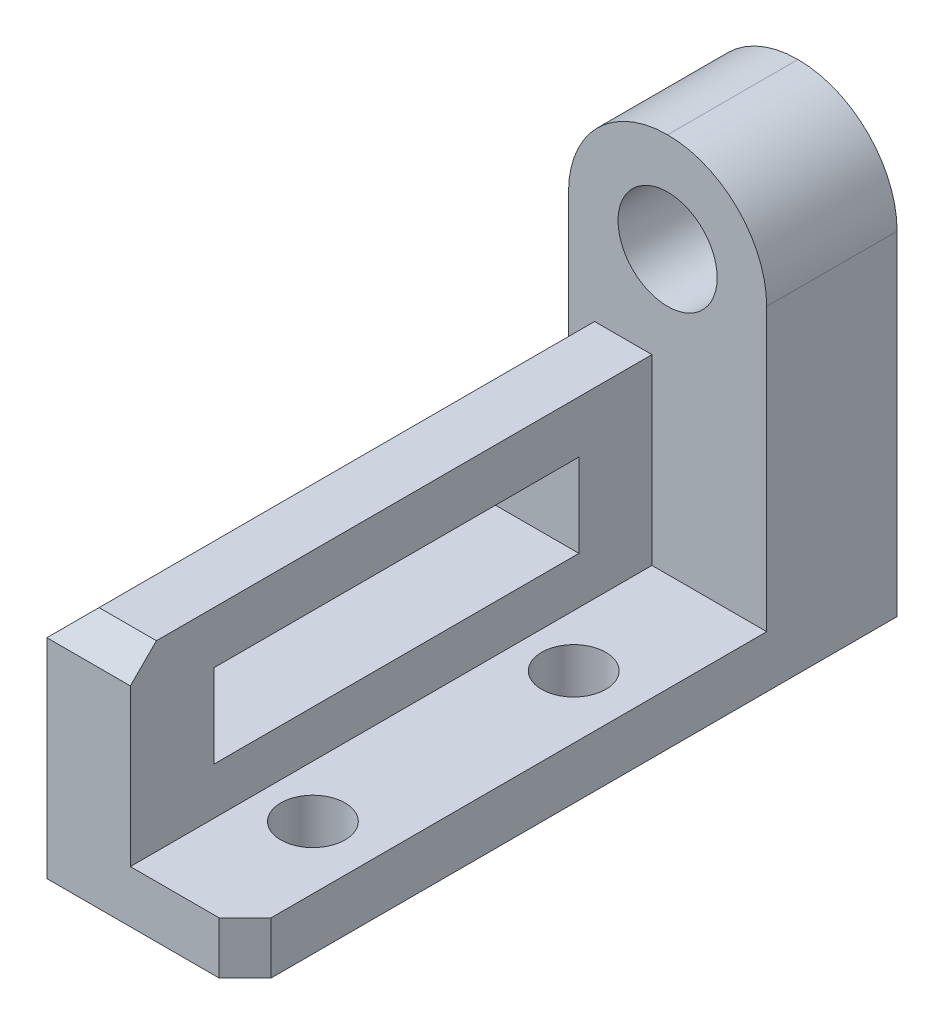
ISO-10303-21;
HEADER;
FILE_DESCRIPTION(('STEP AP214'),'2;1');
FILE_NAME('part.step','',(''),(''),'','','');
FILE_SCHEMA(('AUTOMOTIVE_DESIGN { 1 0 10303 214 1 1 1 1 }'));
ENDSEC;
DATA;
#1=APPLICATION_CONTEXT('core data for automotive mechanical design processes');
#2=APPLICATION_PROTOCOL_DEFINITION('international standard','automotive_design',2000,#1);
#3=PRODUCT_CONTEXT('',#1,'mechanical');
#4=PRODUCT('Part','Part','',(#3));
#5=PRODUCT_RELATED_PRODUCT_CATEGORY('part','',(#4));
#6=PRODUCT_DEFINITION_FORMATION('','',#4);
#7=PRODUCT_DEFINITION_CONTEXT('part definition',#1,'design');
#8=PRODUCT_DEFINITION('design','',#6,#7);
#9=PRODUCT_DEFINITION_SHAPE('','',#8);
#10=(LENGTH_UNIT() NAMED_UNIT(*) SI_UNIT(.MILLI.,.METRE.));
#11=(NAMED_UNIT(*) PLANE_ANGLE_UNIT() SI_UNIT($,.RADIAN.));
#12=(NAMED_UNIT(*) SI_UNIT($,.STERADIAN.) SOLID_ANGLE_UNIT());
#13=UNCERTAINTY_MEASURE_WITH_UNIT(LENGTH_MEASURE(1.E-05),#10,'distance_accuracy_value','');
#14=(GEOMETRIC_REPRESENTATION_CONTEXT(3) GLOBAL_UNCERTAINTY_ASSIGNED_CONTEXT((#13)) GLOBAL_UNIT_ASSIGNED_CONTEXT((#10,
#11,#12)) REPRESENTATION_CONTEXT('',''));
#15=CARTESIAN_POINT('',(0.,0.,0.));
#16=DIRECTION('',(0.,0.,1.));
#17=DIRECTION('',(1.,0.,0.));
#18=AXIS2_PLACEMENT_3D('',#15,#16,#17);
#19=CARTESIAN_POINT('',(38.,10.,-100.));
#20=DIRECTION('',(0.,0.,-1.));
#21=DIRECTION('',(-1.,0.,0.));
#22=AXIS2_PLACEMENT_3D('',#19,#20,#21);
#23=PLANE('',#22);
#24=CARTESIAN_POINT('',(19.,64.,-100.));
#25=DIRECTION('',(0.,0.,1.));
#26=DIRECTION('',(1.,0.,0.));
#27=AXIS2_PLACEMENT_3D('',#24,#25,#26);
#28=CIRCLE('',#27,9.5);
#29=CARTESIAN_POINT('',(28.5,64.,-100.));
#30=VERTEX_POINT('',#29);
#31=EDGE_CURVE('E171',#30,#30,#28,.T.);
#32=ORIENTED_EDGE('',*,*,#31,.F.);
#33=EDGE_LOOP('',(#32));
#34=FACE_BOUND('',#33,.T.);
#35=CARTESIAN_POINT('',(19.,64.,-100.));
#36=DIRECTION('',(0.,0.,-1.));
#37=DIRECTION('',(-1.,0.,0.));
#38=AXIS2_PLACEMENT_3D('',#35,#36,#37);
#39=CIRCLE('',#38,19.);
#40=CARTESIAN_POINT('',(38.,64.,-100.));
#41=VERTEX_POINT('',#40);
#42=CARTESIAN_POINT('',(19.,83.,-100.));
#43=VERTEX_POINT('',#42);
#44=EDGE_CURVE('E259',#41,#43,#39,.F.);
#45=ORIENTED_EDGE('',*,*,#44,.T.);
#46=CARTESIAN_POINT('',(19.,64.,-100.));
#47=DIRECTION('',(0.,0.,-1.));
#48=DIRECTION('',(-1.,0.,0.));
#49=AXIS2_PLACEMENT_3D('',#46,#47,#48);
#50=CIRCLE('',#49,19.);
#51=CARTESIAN_POINT('',(0.,64.,-100.));
#52=VERTEX_POINT('',#51);
#53=EDGE_CURVE('E263',#43,#52,#50,.F.);
#54=ORIENTED_EDGE('',*,*,#53,.T.);
#55=DIRECTION('',(0.,-1.,0.));
#56=VECTOR('',#55,1.);
#57=CARTESIAN_POINT('',(0.,10.,-100.));
#58=LINE('',#57,#56);
#59=CARTESIAN_POINT('',(0.,40.,-100.));
#60=VERTEX_POINT('',#59);
#61=EDGE_CURVE('E207',#52,#60,#58,.T.);
#62=ORIENTED_EDGE('',*,*,#61,.T.);
#63=DIRECTION('',(0.707106781186549,0.707106781186546,0.));
#64=VECTOR('',#63,1.);
#65=CARTESIAN_POINT('',(4.00000000000011,44.0000000000001,-100.));
#66=LINE('',#65,#64);
#67=CARTESIAN_POINT('',(5.00000000000006,45.,-100.));
#68=VERTEX_POINT('',#67);
#69=EDGE_CURVE('E260',#60,#68,#66,.T.);
#70=ORIENTED_EDGE('',*,*,#69,.T.);
#71=DIRECTION('',(-1.,0.,0.));
#72=VECTOR('',#71,1.);
#73=CARTESIAN_POINT('',(0.,45.,-100.));
#74=LINE('',#73,#72);
#75=CARTESIAN_POINT('',(16.,45.,-100.));
#76=VERTEX_POINT('',#75);
#77=EDGE_CURVE('E196',#76,#68,#74,.T.);
#78=ORIENTED_EDGE('',*,*,#77,.F.);
#79=DIRECTION('',(0.,1.,0.));
#80=VECTOR('',#79,1.);
#81=CARTESIAN_POINT('',(16.,45.,-100.));
#82=LINE('',#81,#80);
#83=CARTESIAN_POINT('',(16.,10.,-100.));
#84=VERTEX_POINT('',#83);
#85=EDGE_CURVE('E191',#84,#76,#82,.T.);
#86=ORIENTED_EDGE('',*,*,#85,.F.);
#87=DIRECTION('',(-1.,0.,0.));
#88=VECTOR('',#87,1.);
#89=CARTESIAN_POINT('',(38.,10.,-100.));
#90=LINE('',#89,#88);
#91=CARTESIAN_POINT('',(38.,10.,-100.));
#92=VERTEX_POINT('',#91);
#93=EDGE_CURVE('E230',#92,#84,#90,.T.);
#94=ORIENTED_EDGE('',*,*,#93,.F.);
#95=DIRECTION('',(0.,-1.,0.));
#96=VECTOR('',#95,1.);
#97=CARTESIAN_POINT('',(38.,10.,-100.));
#98=LINE('',#97,#96);
#99=EDGE_CURVE('E215',#41,#92,#98,.T.);
#100=ORIENTED_EDGE('',*,*,#99,.F.);
#101=EDGE_LOOP('',(#45,#54,#62,#70,#78,#86,#94,#100));
#102=FACE_BOUND('',#101,.T.);
#103=ADVANCED_FACE('F41',(#34,#102),#23,.F.);
#104=CARTESIAN_POINT('',(38.,10.,0.));
#105=DIRECTION('',(0.,-1.,0.));
#106=DIRECTION('',(0.,0.,-1.));
#107=AXIS2_PLACEMENT_3D('',#104,#105,#106);
#108=PLANE('',#107);
#109=CARTESIAN_POINT('',(26.,10.,-75.));
#110=DIRECTION('',(0.,1.,0.));
#111=DIRECTION('',(0.,0.,1.));
#112=AXIS2_PLACEMENT_3D('',#109,#110,#111);
#113=CIRCLE('',#112,6.15885509382051);
#114=CARTESIAN_POINT('',(26.,10.,-68.8411449061795));
#115=VERTEX_POINT('',#114);
#116=EDGE_CURVE('E516',#115,#115,#113,.T.);
#117=ORIENTED_EDGE('',*,*,#116,.F.);
#118=EDGE_LOOP('',(#117));
#119=FACE_BOUND('',#118,.T.);
#120=CARTESIAN_POINT('',(26.,10.,-25.));
#121=DIRECTION('',(0.,1.,0.));
#122=DIRECTION('',(0.,0.,1.));
#123=AXIS2_PLACEMENT_3D('',#120,#121,#122);
#124=CIRCLE('',#123,6.15885509382051);
#125=CARTESIAN_POINT('',(26.,10.,-18.8411449061795));
#126=VERTEX_POINT('',#125);
#127=EDGE_CURVE('E524',#126,#126,#124,.T.);
#128=ORIENTED_EDGE('',*,*,#127,.F.);
#129=EDGE_LOOP('',(#128));
#130=FACE_BOUND('',#129,.T.);
#131=DIRECTION('',(-1.,0.,0.));
#132=VECTOR('',#131,1.);
#133=CARTESIAN_POINT('',(38.,10.,0.));
#134=LINE('',#133,#132);
#135=CARTESIAN_POINT('',(33.,10.,0.));
#136=VERTEX_POINT('',#135);
#137=CARTESIAN_POINT('',(16.,10.,0.));
#138=VERTEX_POINT('',#137);
#139=EDGE_CURVE('E220',#136,#138,#134,.T.);
#140=ORIENTED_EDGE('',*,*,#139,.F.);
#141=DIRECTION('',(-0.707106781186549,0.,0.707106781186547));
#142=VECTOR('',#141,1.);
#143=CARTESIAN_POINT('',(38.,10.,-5.00000000000002));
#144=LINE('',#143,#142);
#145=CARTESIAN_POINT('',(38.,10.,-5.00000000000002));
#146=VERTEX_POINT('',#145);
#147=EDGE_CURVE('E241',#136,#146,#144,.F.);
#148=ORIENTED_EDGE('',*,*,#147,.T.);
#149=DIRECTION('',(0.,0.,1.));
#150=VECTOR('',#149,1.);
#151=CARTESIAN_POINT('',(38.,10.,0.));
#152=LINE('',#151,#150);
#153=EDGE_CURVE('E212',#92,#146,#152,.T.);
#154=ORIENTED_EDGE('',*,*,#153,.F.);
#155=ORIENTED_EDGE('',*,*,#93,.T.);
#156=DIRECTION('',(0.,0.,-1.));
#157=VECTOR('',#156,1.);
#158=CARTESIAN_POINT('',(16.,10.,38.4837628097877));
#159=LINE('',#158,#157);
#160=EDGE_CURVE('E195',#138,#84,#159,.T.);
#161=ORIENTED_EDGE('',*,*,#160,.F.);
#162=EDGE_LOOP('',(#140,#148,#154,#155,#161));
#163=FACE_BOUND('',#162,.T.);
#164=ADVANCED_FACE('F306',(#119,#130,#163),#108,.F.);
#165=CARTESIAN_POINT('',(38.,0.,0.));
#166=DIRECTION('',(0.,0.,-1.));
#167=DIRECTION('',(-1.,0.,0.));
#168=AXIS2_PLACEMENT_3D('',#165,#166,#167);
#169=PLANE('',#168);
#170=DIRECTION('',(-1.,0.,0.));
#171=VECTOR('',#170,1.);
#172=CARTESIAN_POINT('',(38.,0.,0.));
#173=LINE('',#172,#171);
#174=CARTESIAN_POINT('',(33.,0.,0.));
#175=VERTEX_POINT('',#174);
#176=CARTESIAN_POINT('',(0.,0.,0.));
#177=VERTEX_POINT('',#176);
#178=EDGE_CURVE('E232',#175,#177,#173,.T.);
#179=ORIENTED_EDGE('',*,*,#178,.F.);
#180=DIRECTION('',(0.,1.,0.));
#181=VECTOR('',#180,1.);
#182=CARTESIAN_POINT('',(33.,0.,0.));
#183=LINE('',#182,#181);
#184=EDGE_CURVE('E243',#175,#136,#183,.T.);
#185=ORIENTED_EDGE('',*,*,#184,.T.);
#186=ORIENTED_EDGE('',*,*,#139,.T.);
#187=DIRECTION('',(0.,-1.,0.));
#188=VECTOR('',#187,1.);
#189=CARTESIAN_POINT('',(16.,45.,0.));
#190=LINE('',#189,#188);
#191=CARTESIAN_POINT('',(16.,40.,0.));
#192=VERTEX_POINT('',#191);
#193=EDGE_CURVE('E193',#192,#138,#190,.T.);
#194=ORIENTED_EDGE('',*,*,#193,.F.);
#195=DIRECTION('',(-1.,0.,0.));
#196=VECTOR('',#195,1.);
#197=CARTESIAN_POINT('',(38.,40.,0.));
#198=LINE('',#197,#196);
#199=CARTESIAN_POINT('',(0.,40.,0.));
#200=VERTEX_POINT('',#199);
#201=EDGE_CURVE('E242',#192,#200,#198,.T.);
#202=ORIENTED_EDGE('',*,*,#201,.T.);
#203=DIRECTION('',(0.,-1.,0.));
#204=VECTOR('',#203,1.);
#205=CARTESIAN_POINT('',(0.,0.,0.));
#206=LINE('',#205,#204);
#207=EDGE_CURVE('E192',#200,#177,#206,.T.);
#208=ORIENTED_EDGE('',*,*,#207,.T.);
#209=EDGE_LOOP('',(#179,#185,#186,#194,#202,#208));
#210=FACE_BOUND('',#209,.T.);
#211=ADVANCED_FACE('F325',(#210),#169,.F.);
#212=CARTESIAN_POINT('',(38.,0.,0.));
#213=DIRECTION('',(0.,1.,0.));
#214=DIRECTION('',(0.,0.,1.));
#215=AXIS2_PLACEMENT_3D('',#212,#213,#214);
#216=PLANE('',#215);
#217=CARTESIAN_POINT('',(26.,0.,-75.));
#218=DIRECTION('',(0.,1.,0.));
#219=DIRECTION('',(0.,0.,1.));
#220=AXIS2_PLACEMENT_3D('',#217,#218,#219);
#221=CIRCLE('',#220,6.15885509382051);
#222=CARTESIAN_POINT('',(26.,0.,-68.8411449061795));
#223=VERTEX_POINT('',#222);
#224=EDGE_CURVE('E520',#223,#223,#221,.T.);
#225=ORIENTED_EDGE('',*,*,#224,.T.);
#226=EDGE_LOOP('',(#225));
#227=FACE_BOUND('',#226,.T.);
#228=CARTESIAN_POINT('',(26.,0.,-25.));
#229=DIRECTION('',(0.,1.,0.));
#230=DIRECTION('',(0.,0.,1.));
#231=AXIS2_PLACEMENT_3D('',#228,#229,#230);
#232=CIRCLE('',#231,6.15885509382051);
#233=CARTESIAN_POINT('',(26.,0.,-18.8411449061795));
#234=VERTEX_POINT('',#233);
#235=EDGE_CURVE('E521',#234,#234,#232,.T.);
#236=ORIENTED_EDGE('',*,*,#235,.T.);
#237=EDGE_LOOP('',(#236));
#238=FACE_BOUND('',#237,.T.);
#239=DIRECTION('',(0.,0.,-1.));
#240=VECTOR('',#239,1.);
#241=CARTESIAN_POINT('',(38.,0.,0.));
#242=LINE('',#241,#240);
#243=CARTESIAN_POINT('',(38.,0.,-5.00000000000002));
#244=VERTEX_POINT('',#243);
#245=CARTESIAN_POINT('',(38.,0.,-125.));
#246=VERTEX_POINT('',#245);
#247=EDGE_CURVE('E206',#244,#246,#242,.T.);
#248=ORIENTED_EDGE('',*,*,#247,.F.);
#249=DIRECTION('',(0.707106781186549,0.,-0.707106781186547));
#250=VECTOR('',#249,1.);
#251=CARTESIAN_POINT('',(38.,0.,-5.00000000000002));
#252=LINE('',#251,#250);
#253=EDGE_CURVE('E239',#244,#175,#252,.F.);
#254=ORIENTED_EDGE('',*,*,#253,.T.);
#255=ORIENTED_EDGE('',*,*,#178,.T.);
#256=DIRECTION('',(0.,0.,-1.));
#257=VECTOR('',#256,1.);
#258=CARTESIAN_POINT('',(0.,0.,0.));
#259=LINE('',#258,#257);
#260=CARTESIAN_POINT('',(0.,0.,-125.));
#261=VERTEX_POINT('',#260);
#262=EDGE_CURVE('E218',#177,#261,#259,.T.);
#263=ORIENTED_EDGE('',*,*,#262,.T.);
#264=DIRECTION('',(-1.,0.,0.));
#265=VECTOR('',#264,1.);
#266=CARTESIAN_POINT('',(38.,0.,-125.));
#267=LINE('',#266,#265);
#268=EDGE_CURVE('E226',#246,#261,#267,.T.);
#269=ORIENTED_EDGE('',*,*,#268,.F.);
#270=EDGE_LOOP('',(#248,#254,#255,#263,#269));
#271=FACE_BOUND('',#270,.T.);
#272=ADVANCED_FACE('F317',(#227,#238,#271),#216,.F.);
#273=CARTESIAN_POINT('',(38.,0.,-125.));
#274=DIRECTION('',(0.,0.,1.));
#275=DIRECTION('',(1.,0.,0.));
#276=AXIS2_PLACEMENT_3D('',#273,#274,#275);
#277=PLANE('',#276);
#278=CARTESIAN_POINT('',(19.,64.,-125.));
#279=DIRECTION('',(0.,0.,1.));
#280=DIRECTION('',(1.,0.,0.));
#281=AXIS2_PLACEMENT_3D('',#278,#279,#280);
#282=CIRCLE('',#281,9.5);
#283=CARTESIAN_POINT('',(28.5,64.,-125.));
#284=VERTEX_POINT('',#283);
#285=EDGE_CURVE('E185',#284,#284,#282,.T.);
#286=ORIENTED_EDGE('',*,*,#285,.T.);
#287=EDGE_LOOP('',(#286));
#288=FACE_BOUND('',#287,.T.);
#289=DIRECTION('',(0.,1.,0.));
#290=VECTOR('',#289,1.);
#291=CARTESIAN_POINT('',(0.,0.,-125.));
#292=LINE('',#291,#290);
#293=CARTESIAN_POINT('',(0.,64.,-125.));
#294=VERTEX_POINT('',#293);
#295=EDGE_CURVE('E222',#261,#294,#292,.T.);
#296=ORIENTED_EDGE('',*,*,#295,.T.);
#297=CARTESIAN_POINT('',(19.,64.,-125.));
#298=DIRECTION('',(0.,0.,1.));
#299=DIRECTION('',(1.,0.,0.));
#300=AXIS2_PLACEMENT_3D('',#297,#298,#299);
#301=CIRCLE('',#300,19.);
#302=CARTESIAN_POINT('',(19.,83.,-125.));
#303=VERTEX_POINT('',#302);
#304=EDGE_CURVE('E49',#294,#303,#301,.F.);
#305=ORIENTED_EDGE('',*,*,#304,.T.);
#306=CARTESIAN_POINT('',(19.,64.,-125.));
#307=DIRECTION('',(0.,0.,1.));
#308=DIRECTION('',(1.,0.,0.));
#309=AXIS2_PLACEMENT_3D('',#306,#307,#308);
#310=CIRCLE('',#309,19.);
#311=CARTESIAN_POINT('',(38.,64.,-125.));
#312=VERTEX_POINT('',#311);
#313=EDGE_CURVE('E268',#303,#312,#310,.F.);
#314=ORIENTED_EDGE('',*,*,#313,.T.);
#315=DIRECTION('',(0.,1.,0.));
#316=VECTOR('',#315,1.);
#317=CARTESIAN_POINT('',(38.,0.,-125.));
#318=LINE('',#317,#316);
#319=EDGE_CURVE('E208',#246,#312,#318,.T.);
#320=ORIENTED_EDGE('',*,*,#319,.F.);
#321=ORIENTED_EDGE('',*,*,#268,.T.);
#322=EDGE_LOOP('',(#296,#305,#314,#320,#321));
#323=FACE_BOUND('',#322,.T.);
#324=ADVANCED_FACE('F275',(#288,#323),#277,.F.);
#325=CARTESIAN_POINT('',(38.,0.,0.));
#326=DIRECTION('',(-1.,0.,0.));
#327=DIRECTION('',(0.,0.,1.));
#328=AXIS2_PLACEMENT_3D('',#325,#326,#327);
#329=PLANE('',#328);
#330=ORIENTED_EDGE('',*,*,#319,.T.);
#331=DIRECTION('',(0.,0.,1.));
#332=VECTOR('',#331,1.);
#333=CARTESIAN_POINT('',(38.,64.,0.));
#334=LINE('',#333,#332);
#335=EDGE_CURVE('E11',#312,#41,#334,.T.);
#336=ORIENTED_EDGE('',*,*,#335,.T.);
#337=ORIENTED_EDGE('',*,*,#99,.T.);
#338=ORIENTED_EDGE('',*,*,#153,.T.);
#339=DIRECTION('',(0.,-1.,0.));
#340=VECTOR('',#339,1.);
#341=CARTESIAN_POINT('',(38.,0.,-5.00000000000002));
#342=LINE('',#341,#340);
#343=EDGE_CURVE('E237',#146,#244,#342,.T.);
#344=ORIENTED_EDGE('',*,*,#343,.T.);
#345=ORIENTED_EDGE('',*,*,#247,.T.);
#346=EDGE_LOOP('',(#330,#336,#337,#338,#344,#345));
#347=FACE_BOUND('',#346,.T.);
#348=ADVANCED_FACE('F315',(#347),#329,.F.);
#349=CARTESIAN_POINT('',(0.,0.,0.));
#350=DIRECTION('',(-1.,0.,0.));
#351=DIRECTION('',(0.,0.,1.));
#352=AXIS2_PLACEMENT_3D('',#349,#350,#351);
#353=PLANE('',#352);
#354=DIRECTION('',(0.,-1.,0.));
#355=VECTOR('',#354,1.);
#356=CARTESIAN_POINT('',(0.,35.,-16.));
#357=LINE('',#356,#355);
#358=CARTESIAN_POINT('',(0.,35.,-16.));
#359=VERTEX_POINT('',#358);
#360=CARTESIAN_POINT('',(0.,19.,-16.));
#361=VERTEX_POINT('',#360);
#362=EDGE_CURVE('E153',#359,#361,#357,.T.);
#363=ORIENTED_EDGE('',*,*,#362,.T.);
#364=DIRECTION('',(0.,0.,-1.));
#365=VECTOR('',#364,1.);
#366=CARTESIAN_POINT('',(0.,19.,-16.));
#367=LINE('',#366,#365);
#368=CARTESIAN_POINT('',(0.,19.,-86.));
#369=VERTEX_POINT('',#368);
#370=EDGE_CURVE('E165',#361,#369,#367,.T.);
#371=ORIENTED_EDGE('',*,*,#370,.T.);
#372=DIRECTION('',(0.,1.,0.));
#373=VECTOR('',#372,1.);
#374=CARTESIAN_POINT('',(0.,35.,-86.));
#375=LINE('',#374,#373);
#376=CARTESIAN_POINT('',(0.,35.,-86.));
#377=VERTEX_POINT('',#376);
#378=EDGE_CURVE('E60',#369,#377,#375,.T.);
#379=ORIENTED_EDGE('',*,*,#378,.T.);
#380=DIRECTION('',(0.,0.,1.));
#381=VECTOR('',#380,1.);
#382=CARTESIAN_POINT('',(0.,35.,-16.));
#383=LINE('',#382,#381);
#384=EDGE_CURVE('E157',#377,#359,#383,.T.);
#385=ORIENTED_EDGE('',*,*,#384,.T.);
#386=EDGE_LOOP('',(#363,#371,#379,#385));
#387=FACE_BOUND('',#386,.T.);
#388=ORIENTED_EDGE('',*,*,#61,.F.);
#389=DIRECTION('',(0.,0.,1.));
#390=VECTOR('',#389,1.);
#391=CARTESIAN_POINT('',(0.,64.,-125.));
#392=LINE('',#391,#390);
#393=EDGE_CURVE('E264',#52,#294,#392,.F.);
#394=ORIENTED_EDGE('',*,*,#393,.T.);
#395=ORIENTED_EDGE('',*,*,#295,.F.);
#396=ORIENTED_EDGE('',*,*,#262,.F.);
#397=ORIENTED_EDGE('',*,*,#207,.F.);
#398=DIRECTION('',(0.,0.,-1.));
#399=VECTOR('',#398,1.);
#400=CARTESIAN_POINT('',(0.,40.,-100.));
#401=LINE('',#400,#399);
#402=EDGE_CURVE('E255',#200,#60,#401,.T.);
#403=ORIENTED_EDGE('',*,*,#402,.T.);
#404=EDGE_LOOP('',(#388,#394,#395,#396,#397,#403));
#405=FACE_BOUND('',#404,.T.);
#406=ADVANCED_FACE('F167',(#387,#405),#353,.T.);
#407=CARTESIAN_POINT('',(0.,45.,38.4837628097877));
#408=DIRECTION('',(0.,-1.,0.));
#409=DIRECTION('',(0.,0.,-1.));
#410=AXIS2_PLACEMENT_3D('',#407,#408,#409);
#411=PLANE('',#410);
#412=DIRECTION('',(0.,0.,1.));
#413=VECTOR('',#412,1.);
#414=CARTESIAN_POINT('',(5.00000000000006,45.,0.));
#415=LINE('',#414,#413);
#416=CARTESIAN_POINT('',(5.00000000000006,45.,-5.00000000000006));
#417=VERTEX_POINT('',#416);
#418=EDGE_CURVE('E249',#68,#417,#415,.T.);
#419=ORIENTED_EDGE('',*,*,#418,.T.);
#420=DIRECTION('',(1.,0.,0.));
#421=VECTOR('',#420,1.);
#422=CARTESIAN_POINT('',(0.,45.,-5.00000000000006));
#423=LINE('',#422,#421);
#424=CARTESIAN_POINT('',(16.,45.,-5.00000000000006));
#425=VERTEX_POINT('',#424);
#426=EDGE_CURVE('E250',#417,#425,#423,.T.);
#427=ORIENTED_EDGE('',*,*,#426,.T.);
#428=DIRECTION('',(0.,0.,-1.));
#429=VECTOR('',#428,1.);
#430=CARTESIAN_POINT('',(16.,45.,38.4837628097877));
#431=LINE('',#430,#429);
#432=EDGE_CURVE('E205',#425,#76,#431,.T.);
#433=ORIENTED_EDGE('',*,*,#432,.T.);
#434=ORIENTED_EDGE('',*,*,#77,.T.);
#435=EDGE_LOOP('',(#419,#427,#433,#434));
#436=FACE_BOUND('',#435,.T.);
#437=ADVANCED_FACE('F300',(#436),#411,.F.);
#438=CARTESIAN_POINT('',(16.,45.,38.4837628097877));
#439=DIRECTION('',(-1.,0.,0.));
#440=DIRECTION('',(0.,-1.,0.));
#441=AXIS2_PLACEMENT_3D('',#438,#439,#440);
#442=PLANE('',#441);
#443=DIRECTION('',(0.,0.,-1.));
#444=VECTOR('',#443,1.);
#445=CARTESIAN_POINT('',(16.,19.,-16.));
#446=LINE('',#445,#444);
#447=CARTESIAN_POINT('',(16.,19.,-16.));
#448=VERTEX_POINT('',#447);
#449=CARTESIAN_POINT('',(16.,19.,-86.));
#450=VERTEX_POINT('',#449);
#451=EDGE_CURVE('E182',#448,#450,#446,.T.);
#452=ORIENTED_EDGE('',*,*,#451,.F.);
#453=DIRECTION('',(0.,-1.,0.));
#454=VECTOR('',#453,1.);
#455=CARTESIAN_POINT('',(16.,35.,-16.));
#456=LINE('',#455,#454);
#457=CARTESIAN_POINT('',(16.,35.,-16.));
#458=VERTEX_POINT('',#457);
#459=EDGE_CURVE('E61',#458,#448,#456,.T.);
#460=ORIENTED_EDGE('',*,*,#459,.F.);
#461=DIRECTION('',(0.,0.,1.));
#462=VECTOR('',#461,1.);
#463=CARTESIAN_POINT('',(16.,35.,-16.));
#464=LINE('',#463,#462);
#465=CARTESIAN_POINT('',(16.,35.,-86.));
#466=VERTEX_POINT('',#465);
#467=EDGE_CURVE('E166',#466,#458,#464,.T.);
#468=ORIENTED_EDGE('',*,*,#467,.F.);
#469=DIRECTION('',(0.,1.,0.));
#470=VECTOR('',#469,1.);
#471=CARTESIAN_POINT('',(16.,35.,-86.));
#472=LINE('',#471,#470);
#473=EDGE_CURVE('E175',#450,#466,#472,.T.);
#474=ORIENTED_EDGE('',*,*,#473,.F.);
#475=EDGE_LOOP('',(#452,#460,#468,#474));
#476=FACE_BOUND('',#475,.T.);
#477=ORIENTED_EDGE('',*,*,#432,.F.);
#478=DIRECTION('',(0.,0.707106781186546,-0.707106781186549));
#479=VECTOR('',#478,1.);
#480=CARTESIAN_POINT('',(16.,45.,-5.00000000000006));
#481=LINE('',#480,#479);
#482=EDGE_CURVE('E252',#425,#192,#481,.F.);
#483=ORIENTED_EDGE('',*,*,#482,.T.);
#484=ORIENTED_EDGE('',*,*,#193,.T.);
#485=ORIENTED_EDGE('',*,*,#160,.T.);
#486=ORIENTED_EDGE('',*,*,#85,.T.);
#487=EDGE_LOOP('',(#477,#483,#484,#485,#486));
#488=FACE_BOUND('',#487,.T.);
#489=ADVANCED_FACE('F303',(#476,#488),#442,.F.);
#490=CARTESIAN_POINT('',(38.,0.,-5.00000000000002));
#491=DIRECTION('',(-0.707106781186546,0.,-0.707106781186548));
#492=DIRECTION('',(0.,-1.,0.));
#493=AXIS2_PLACEMENT_3D('',#490,#491,#492);
#494=PLANE('',#493);
#495=ORIENTED_EDGE('',*,*,#147,.F.);
#496=ORIENTED_EDGE('',*,*,#184,.F.);
#497=ORIENTED_EDGE('',*,*,#253,.F.);
#498=ORIENTED_EDGE('',*,*,#343,.F.);
#499=EDGE_LOOP('',(#495,#496,#497,#498));
#500=FACE_BOUND('',#499,.T.);
#501=ADVANCED_FACE('F312',(#500),#494,.F.);
#502=CARTESIAN_POINT('',(0.,40.,0.));
#503=DIRECTION('',(-0.707106781186546,0.707106781186549,0.));
#504=DIRECTION('',(0.,0.,1.));
#505=AXIS2_PLACEMENT_3D('',#502,#503,#504);
#506=PLANE('',#505);
#507=ORIENTED_EDGE('',*,*,#69,.F.);
#508=ORIENTED_EDGE('',*,*,#402,.F.);
#509=DIRECTION('',(-0.577350269189627,-0.577350269189624,0.577350269189627));
#510=VECTOR('',#509,1.);
#511=CARTESIAN_POINT('',(0.,40.,0.));
#512=LINE('',#511,#510);
#513=EDGE_CURVE('E200',#417,#200,#512,.T.);
#514=ORIENTED_EDGE('',*,*,#513,.F.);
#515=ORIENTED_EDGE('',*,*,#418,.F.);
#516=EDGE_LOOP('',(#507,#508,#514,#515));
#517=FACE_BOUND('',#516,.T.);
#518=ADVANCED_FACE('F294',(#517),#506,.T.);
#519=CARTESIAN_POINT('',(0.,45.,-5.00000000000006));
#520=DIRECTION('',(0.,-0.707106781186549,-0.707106781186546));
#521=DIRECTION('',(1.,0.,0.));
#522=AXIS2_PLACEMENT_3D('',#519,#520,#521);
#523=PLANE('',#522);
#524=ORIENTED_EDGE('',*,*,#513,.T.);
#525=ORIENTED_EDGE('',*,*,#201,.F.);
#526=ORIENTED_EDGE('',*,*,#482,.F.);
#527=ORIENTED_EDGE('',*,*,#426,.F.);
#528=EDGE_LOOP('',(#524,#525,#526,#527));
#529=FACE_BOUND('',#528,.T.);
#530=ADVANCED_FACE('F324',(#529),#523,.F.);
#531=CARTESIAN_POINT('',(19.,64.,0.));
#532=DIRECTION('',(0.,0.,1.));
#533=DIRECTION('',(1.,0.,0.));
#534=AXIS2_PLACEMENT_3D('',#531,#532,#533);
#535=CYLINDRICAL_SURFACE('',#534,19.);
#536=ORIENTED_EDGE('',*,*,#335,.F.);
#537=ORIENTED_EDGE('',*,*,#313,.F.);
#538=DIRECTION('',(0.,0.,1.));
#539=VECTOR('',#538,1.);
#540=CARTESIAN_POINT('',(19.,83.,-125.));
#541=LINE('',#540,#539);
#542=EDGE_CURVE('E44',#43,#303,#541,.F.);
#543=ORIENTED_EDGE('',*,*,#542,.F.);
#544=ORIENTED_EDGE('',*,*,#44,.F.);
#545=EDGE_LOOP('',(#536,#537,#543,#544));
#546=FACE_BOUND('',#545,.T.);
#547=ADVANCED_FACE('F43',(#546),#535,.T.);
#548=CARTESIAN_POINT('',(19.,64.,-125.));
#549=DIRECTION('',(0.,0.,-1.));
#550=DIRECTION('',(-1.,0.,0.));
#551=AXIS2_PLACEMENT_3D('',#548,#549,#550);
#552=CYLINDRICAL_SURFACE('',#551,19.);
#553=ORIENTED_EDGE('',*,*,#304,.F.);
#554=ORIENTED_EDGE('',*,*,#393,.F.);
#555=ORIENTED_EDGE('',*,*,#53,.F.);
#556=ORIENTED_EDGE('',*,*,#542,.T.);
#557=EDGE_LOOP('',(#553,#554,#555,#556));
#558=FACE_BOUND('',#557,.T.);
#559=ADVANCED_FACE('F283',(#558),#552,.T.);
#560=CARTESIAN_POINT('',(0.,35.,-16.));
#561=DIRECTION('',(0.,0.,1.));
#562=DIRECTION('',(0.,-1.,0.));
#563=AXIS2_PLACEMENT_3D('',#560,#561,#562);
#564=PLANE('',#563);
#565=ORIENTED_EDGE('',*,*,#459,.T.);
#566=DIRECTION('',(1.,0.,0.));
#567=VECTOR('',#566,1.);
#568=CARTESIAN_POINT('',(0.,19.,-16.));
#569=LINE('',#568,#567);
#570=EDGE_CURVE('E149',#361,#448,#569,.T.);
#571=ORIENTED_EDGE('',*,*,#570,.F.);
#572=ORIENTED_EDGE('',*,*,#362,.F.);
#573=DIRECTION('',(1.,0.,0.));
#574=VECTOR('',#573,1.);
#575=CARTESIAN_POINT('',(0.,35.,-16.));
#576=LINE('',#575,#574);
#577=EDGE_CURVE('E187',#359,#458,#576,.T.);
#578=ORIENTED_EDGE('',*,*,#577,.T.);
#579=EDGE_LOOP('',(#565,#571,#572,#578));
#580=FACE_BOUND('',#579,.T.);
#581=ADVANCED_FACE('F151',(#580),#564,.F.);
#582=CARTESIAN_POINT('',(0.,35.,-16.));
#583=DIRECTION('',(0.,1.,0.));
#584=DIRECTION('',(-1.,0.,0.));
#585=AXIS2_PLACEMENT_3D('',#582,#583,#584);
#586=PLANE('',#585);
#587=ORIENTED_EDGE('',*,*,#467,.T.);
#588=ORIENTED_EDGE('',*,*,#577,.F.);
#589=ORIENTED_EDGE('',*,*,#384,.F.);
#590=DIRECTION('',(1.,0.,0.));
#591=VECTOR('',#590,1.);
#592=CARTESIAN_POINT('',(0.,35.,-86.));
#593=LINE('',#592,#591);
#594=EDGE_CURVE('E188',#377,#466,#593,.T.);
#595=ORIENTED_EDGE('',*,*,#594,.T.);
#596=EDGE_LOOP('',(#587,#588,#589,#595));
#597=FACE_BOUND('',#596,.T.);
#598=ADVANCED_FACE('F453',(#597),#586,.F.);
#599=CARTESIAN_POINT('',(0.,35.,-86.));
#600=DIRECTION('',(0.,0.,-1.));
#601=DIRECTION('',(-1.,0.,0.));
#602=AXIS2_PLACEMENT_3D('',#599,#600,#601);
#603=PLANE('',#602);
#604=ORIENTED_EDGE('',*,*,#473,.T.);
#605=ORIENTED_EDGE('',*,*,#594,.F.);
#606=ORIENTED_EDGE('',*,*,#378,.F.);
#607=DIRECTION('',(1.,0.,0.));
#608=VECTOR('',#607,1.);
#609=CARTESIAN_POINT('',(0.,19.,-86.));
#610=LINE('',#609,#608);
#611=EDGE_CURVE('E158',#369,#450,#610,.T.);
#612=ORIENTED_EDGE('',*,*,#611,.T.);
#613=EDGE_LOOP('',(#604,#605,#606,#612));
#614=FACE_BOUND('',#613,.T.);
#615=ADVANCED_FACE('F456',(#614),#603,.F.);
#616=CARTESIAN_POINT('',(0.,19.,-16.));
#617=DIRECTION('',(0.,-1.,0.));
#618=DIRECTION('',(1.,0.,0.));
#619=AXIS2_PLACEMENT_3D('',#616,#617,#618);
#620=PLANE('',#619);
#621=ORIENTED_EDGE('',*,*,#451,.T.);
#622=ORIENTED_EDGE('',*,*,#611,.F.);
#623=ORIENTED_EDGE('',*,*,#370,.F.);
#624=ORIENTED_EDGE('',*,*,#570,.T.);
#625=EDGE_LOOP('',(#621,#622,#623,#624));
#626=FACE_BOUND('',#625,.T.);
#627=ADVANCED_FACE('F162',(#626),#620,.F.);
#628=CARTESIAN_POINT('',(19.,64.,-125.));
#629=DIRECTION('',(0.,0.,1.));
#630=DIRECTION('',(1.,0.,0.));
#631=AXIS2_PLACEMENT_3D('',#628,#629,#630);
#632=CYLINDRICAL_SURFACE('',#631,9.5);
#633=ORIENTED_EDGE('',*,*,#285,.F.);
#634=EDGE_LOOP('',(#633));
#635=FACE_BOUND('',#634,.T.);
#636=ORIENTED_EDGE('',*,*,#31,.T.);
#637=EDGE_LOOP('',(#636));
#638=FACE_BOUND('',#637,.T.);
#639=ADVANCED_FACE('F471',(#635,#638),#632,.F.);
#640=CARTESIAN_POINT('',(26.,0.,-25.));
#641=DIRECTION('',(0.,1.,0.));
#642=DIRECTION('',(0.,0.,1.));
#643=AXIS2_PLACEMENT_3D('',#640,#641,#642);
#644=CYLINDRICAL_SURFACE('',#643,6.15885509382051);
#645=ORIENTED_EDGE('',*,*,#235,.F.);
#646=EDGE_LOOP('',(#645));
#647=FACE_BOUND('',#646,.T.);
#648=ORIENTED_EDGE('',*,*,#127,.T.);
#649=EDGE_LOOP('',(#648));
#650=FACE_BOUND('',#649,.T.);
#651=ADVANCED_FACE('F481',(#647,#650),#644,.F.);
#652=CARTESIAN_POINT('',(26.,0.,-75.));
#653=DIRECTION('',(0.,1.,0.));
#654=DIRECTION('',(0.,0.,1.));
#655=AXIS2_PLACEMENT_3D('',#652,#653,#654);
#656=CYLINDRICAL_SURFACE('',#655,6.15885509382051);
#657=ORIENTED_EDGE('',*,*,#224,.F.);
#658=EDGE_LOOP('',(#657));
#659=FACE_BOUND('',#658,.T.);
#660=ORIENTED_EDGE('',*,*,#116,.T.);
#661=EDGE_LOOP('',(#660));
#662=FACE_BOUND('',#661,.T.);
#663=ADVANCED_FACE('F489',(#659,#662),#656,.F.);
#664=CLOSED_SHELL('',(#103,#164,#211,#272,#324,#348,#406,#437,#489,#501,#518,#530,#547,#559,
#581,#598,#615,#627,#639,#651,#663));
#665=MANIFOLD_SOLID_BREP('B2',#664);
#666=ADVANCED_BREP_SHAPE_REPRESENTATION('',(#18,#665),#14);
#667=SHAPE_DEFINITION_REPRESENTATION(#9,#666);
ENDSEC;
END-ISO-10303-21;
